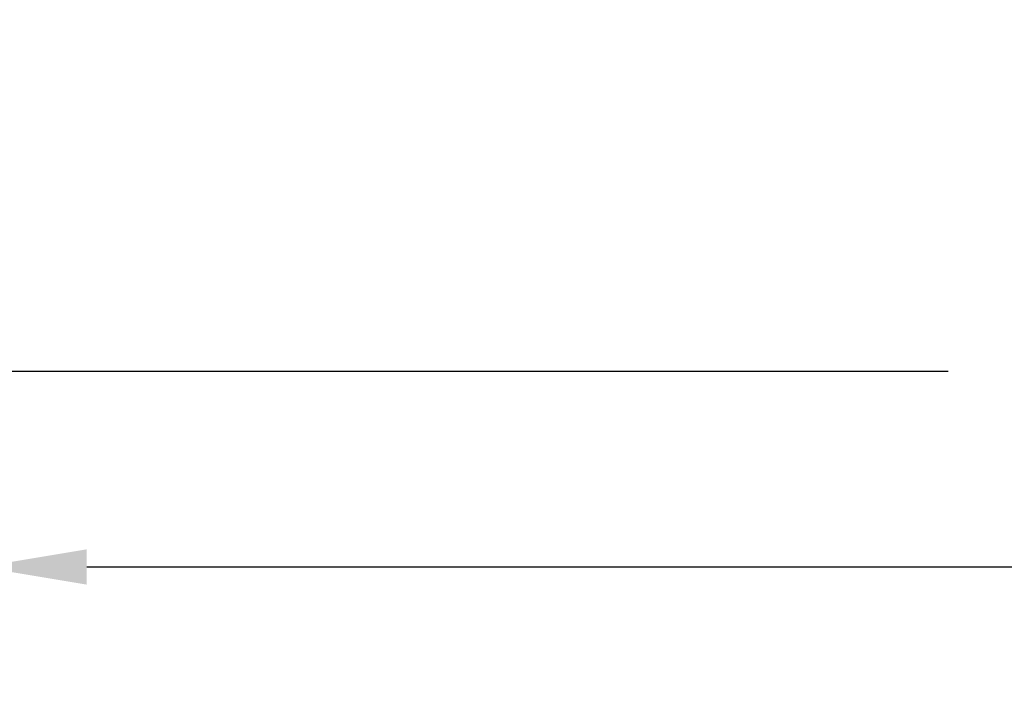
# Model space of a CAD drawing. Units: millimetres. Extents: x 7894 to 8038, y 6851 to 6951.
# Tile 2 of 49: x 7944.854 to 7954.151, y 6858.512 to 6864.931. Entities that reach past the tile are written whole.
import ezdxf

# ---------------------------------------------------------------- set-up
doc = ezdxf.new("R2010")
doc.units = ezdxf.units.MM
doc.layers.add('A-ANNO-DIMS', color=2, linetype='Continuous', lineweight=18)
doc.styles.get("Standard").update_dxf_attribs({"font": 'arial.ttf'})
doc.dimstyles.new('ISO-25', dxfattribs={"dimtxt": 1, "dimasz": 1, "dimexe": 1.25, "dimexo": 0.625, "dimtad": 1, "dimdec": 0, "dimlunit": 4, "dimtxsty": 'Standard', "dimcen": 2.5, "dimclrt": 1, "dimadec": 0, "dimazin": 0, "dimtfac": 1, "dimtdec": 0, "dimtmove": 0, "dimatfit": 3, "dimfxl": 1, "dimarcsym": 0})

# ---------------------------------------------------------------- blocks, each defined once
blk = doc.blocks.new('*D36')
at = {"layer": 'A-ANNO-DIMS', "color": 0, "lineweight": -2, "transparency": 16777216}
for p, q in [((7980.8359, 6877.9586), (7980.8359, 6858.5122)), ((7944.4866, 6864.4359), (7944.4866, 6858.5122)), ((7945.4866, 6859.7622), (7979.8359, 6859.7622))]:
    blk.add_line(p, q, dxfattribs=at)
at = {"layer": 'A-ANNO-DIMS', "color": 0, "transparency": 16777216}
for points in [[(7945.4866, 6859.9288), (7945.4866, 6859.5955), (7944.4866, 6859.7622)], [(7979.8359, 6859.9288), (7979.8359, 6859.5955), (7980.8359, 6859.7622)]]:
    blk.add_solid(points, dxfattribs=at)
at = {"layer": 'Defpoints', "color": 0, "transparency": 16777216}
for p in [(7980.8359, 6878.5836), (7944.4866, 6865.0609), (7980.8359, 6859.7622)]:
    blk.add_point(p, dxfattribs=at)
at = {"layer": 'A-ANNO-DIMS', "color": 1, "transparency": 16777216, "insert": (7962.6613, 6860.9046), "char_height": 1, "attachment_point": 5}
blk.add_mtext('3\'-0 1/2"', dxfattribs=at)
blk = doc.blocks.new('*D37')
at = {"layer": 'A-ANNO-DIMS', "color": 0, "lineweight": -2, "transparency": 16777216}
for p, q in [((7954.9197, 6887.9028), (7941.3891, 6887.9028)), ((7942.6391, 6862.6097), (7942.6391, 6886.9028)), ((7953.6228, 6861.6097), (7941.3891, 6861.6097))]:
    blk.add_line(p, q, dxfattribs=at)
at = {"layer": 'A-ANNO-DIMS', "color": 0, "transparency": 16777216}
for points in [[(7942.4724, 6886.9028), (7942.8057, 6886.9028), (7942.6391, 6887.9028)], [(7942.4724, 6862.6097), (7942.8057, 6862.6097), (7942.6391, 6861.6097)]]:
    blk.add_solid(points, dxfattribs=at)
at = {"layer": 'Defpoints', "color": 0, "transparency": 16777216}
for p in [(7942.6391, 6887.9028), (7955.5447, 6887.9028), (7954.2478, 6861.6097)]:
    blk.add_point(p, dxfattribs=at)
at = {"layer": 'A-ANNO-DIMS', "color": 1, "transparency": 16777216, "insert": (7941.497, 6874.7562), "char_height": 1, "attachment_point": 5, "rotation": 90}
blk.add_mtext('2\'-2 1/2"', dxfattribs=at)

msp = doc.modelspace()

# ---------------------------------------------------------------- dimensions: what is measured, and where the dimension line sits
at = {"layer": 'A-ANNO-DIMS'}
dim = msp.add_linear_dim(base=(7942.6391, 6887.9028), p1=(7954.2478, 6861.6097), p2=(7955.5447, 6887.9028), angle=90, dimstyle='ISO-25', override={"dimdec": 1, "dimlfac": 1, "dimrnd": 0, "dimzin": 1, "dimdsep": 46, "dimlunit": 4, "dimfrac": 2}, dxfattribs=at)
dim.commit()
dim.dimension.update_dxf_attribs({"geometry": '*D37', "text_midpoint": (7941.497, 6874.7562)})
dim = msp.add_linear_dim(base=(7980.8359, 6859.7622), p1=(7944.4866, 6865.0609), p2=(7980.8359, 6878.5836), dimstyle='ISO-25', override={"dimdec": 1, "dimlfac": 1, "dimrnd": 0, "dimzin": 1, "dimdsep": 46, "dimlunit": 4, "dimfrac": 2}, dxfattribs=at)
dim.commit()
dim.dimension.update_dxf_attribs({"geometry": '*D36', "text_midpoint": (7962.6613, 6860.9046)})

doc.saveas('drawing.dxf')
